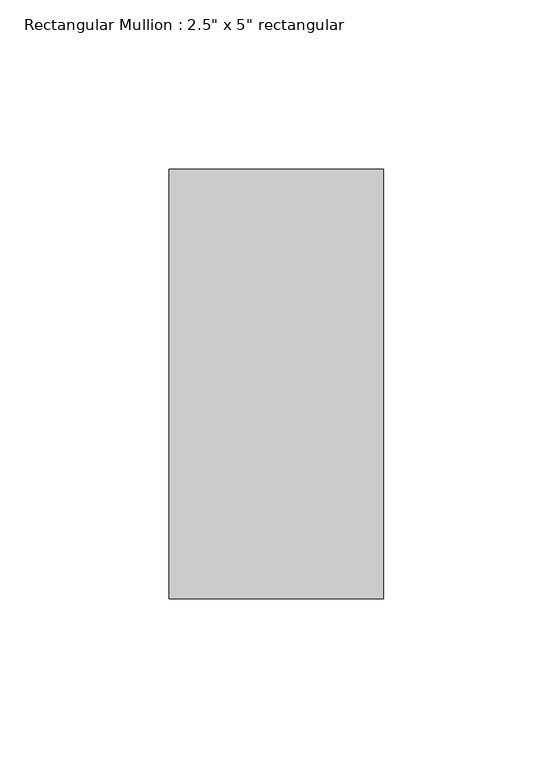
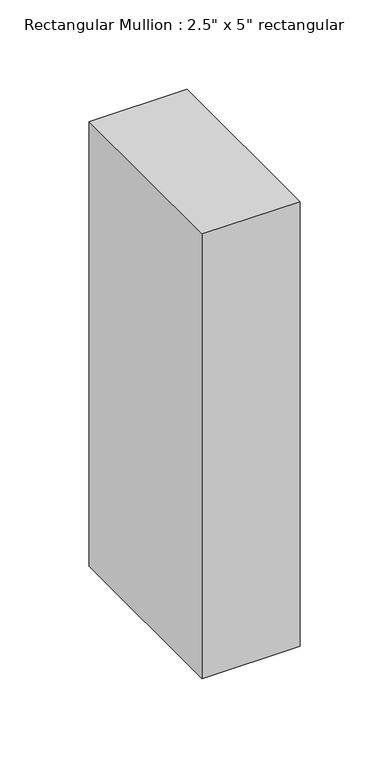
"""IFC4 building model written with IfcOpenShell, lengths in millimetres: member geometry."""

from ifc_helpers import new_model, si_unit, frame, origin, place, context, project, spatial, polyline, outline, extrude, source, transform, mapped, element, save


def member_75d1e245(model_context):
    return source(origin(), model_context, "Body", "SweptSolid", [
        extrude(outline(polyline([(31.75, 63.5), (31.75, -63.5), (-31.75, -63.5), (-31.75, 63.5), (31.75, 63.5)])), frame((0.0, 0.0, -304.8), z_axis=(0.0, 0.0, 1.0), x_axis=(1.0, 0.0, 0.0)), (0.0, 0.0, 1.0), 304.8),
    ])


if __name__ == "__main__":
    model = new_model("IFC4")
    model_context = context("Model", 3, world=origin())
    ifc_project = project(units=[si_unit("LENGTHUNIT", "METRE", prefix="MILLI")], contexts=[model_context])
    site = spatial("IfcSite", under=ifc_project)
    building = spatial("IfcBuilding", under=site)
    placement = place(None, origin())
    member_shape = member_75d1e245(model_context)
    element("IfcMember", 1, ObjectType="Rectangular Mullion : 2.5\" x 5\" rectangular", at=placement, inside=building, context=model_context, shape_type="MappedRepresentation", body=[
        mapped(member_shape, transform((0.0, 0.0, 0.0), x_axis=(1.0, 0.0, 0.0), y_axis=(0.0, 1.0, 0.0), z_axis=(0.0, 0.0, 1.0))),
    ])
    save(model, "model.ifc")

# Revit data of these elements
# Type "Rectangular Mullion : 2.5\" x 5\" rectangular"
#   built-in parameter 1007304 = 0.416667 (stored number, unit not read)
#   built-in parameter 1007301 = 0.104167 (stored number, unit not read)
#   built-in parameter 1007300 = 0.104167 (stored number, unit not read)
